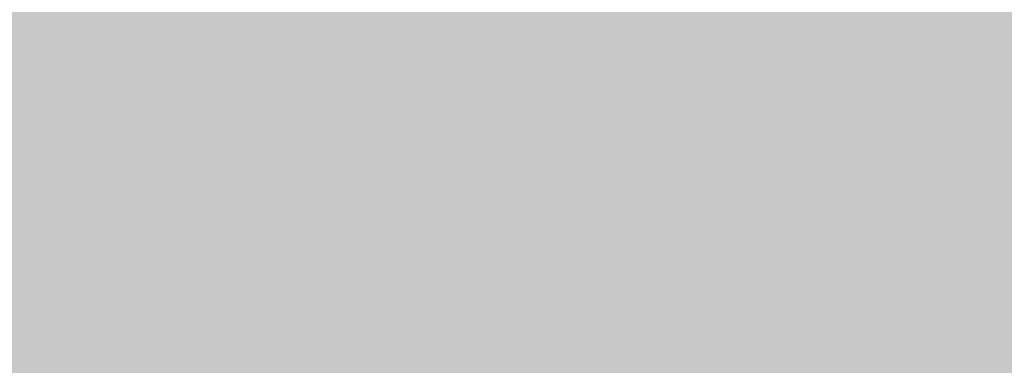
# Model space of a CAD drawing. Units: inches. Extents: x 2091 to 2899, y 967 to 2217.
# Tile 219 of 256: x 2203.2571 to 2203.4104, y 1152.3009 to 1152.3547. Entities that reach past the tile are written whole.
import ezdxf

# ---------------------------------------------------------------- set-up
doc = ezdxf.new("R2010")
doc.units = ezdxf.units.IN
doc.layers.add('A-WALL-PATT', color=141, linetype='Continuous', lineweight=13, true_color=0xadddf7)

msp = doc.modelspace()

# ---------------------------------------------------------------- hatches: boundary and pattern name
at = {"layer": 'A-WALL-PATT'}
h = msp.add_hatch(color=256, dxfattribs=at)
h.dxf.hatch_style = 1
h.paths.add_polyline_path([(2803.1436, 2050.91906), (2203.1436, 2050.91906), (2203.1436, 1090.91906), (2803.1436, 1090.91906)])
h.paths.add_polyline_path([(2635.79885, 1147.54046), (2674.52405, 1147.54046, 0.376086), (2678.52967, 1152.8802), (2678.52967, 1159.55647, 0.333335), (2674.52432, 1163.56185), (2674.52432, 1163.56185), (2674.52432, 1192.93439), (2635.80597, 1192.93439), (2597.08762, 1192.93439), (2597.08762, 1163.56185, 0.333335), (2593.08228, 1159.55647), (2593.08228, 1152.8802, 0.376086), (2597.08789, 1147.54046)], flags=0)
h.paths.add_polyline_path([(2436.01043, 1278.24078, 0.000483), (2435.95264, 1278.21503, -0.001328), (2435.93563, 1278.11169, -0.001711), (2436.11644, 1278.04076, 0.002185)], flags=0)
h.paths.add_polyline_path([(2794.1436, 1143.41906), (2794.1436, 1347.41906), (2543.37017, 1347.41906), (2543.37017, 1351.91906), (2794.1436, 1351.91906), (2794.1436, 1392.71355), (2793.9474, 1392.71355), (2793.9474, 1473.5369), (2794.1436, 1473.5369), (2794.1436, 1531.91906), (2650.1436, 1531.91906), (2650.1436, 1536.41906), (2794.1436, 1536.41906), (2794.1436, 1692.41906), (2609.37561, 1692.41906), (2609.37561, 1644.41906), (2604.87561, 1644.41906), (2604.87561, 1744.91906), (2609.37561, 1744.91906), (2609.37561, 1696.91906), (2794.1436, 1696.91906), (2794.1436, 1780.91906), (2609.6436, 1780.91906), (2493.87561, 1780.91906), (2493.87561, 1785.41906), (2609.6436, 1785.41906), (2794.1436, 1785.41906), (2794.1436, 1847.93882), (2793.95122, 1847.93882), (2793.95122, 1928.76217), (2794.1436, 1928.76217), (2794.1436, 1941.41906), (2614.1436, 1941.41906), (2614.1436, 1821.41906), (2609.6436, 1821.41906), (2609.6436, 1941.41906), (2392.1436, 1941.41906), (2392.1436, 1819.91906), (2387.6436, 1819.91906), (2387.6436, 1941.41906), (2212.1436, 1941.41906), (2212.1436, 1783.91906), (2392.1436, 1783.91906), (2392.1436, 1780.91906), (2212.1436, 1780.91906), (2212.1436, 1629.41906), (2387.6436, 1629.41906), (2387.6436, 1744.91906), (2392.1436, 1744.91906), (2392.1436, 1627.91906), (2317.1436, 1627.91906), (2317.1436, 1551.41906), (2317.1436, 1536.41906), (2459.38359, 1536.41906), (2459.38359, 1602.39648), (2463.88359, 1602.39648), (2463.88359, 1531.91906), (2456.6436, 1531.91906), (2456.6436, 1529.91906), (2452.1436, 1529.91906), (2452.1436, 1531.91906), (2312.6436, 1531.91906), (2312.6436, 1551.41906), (2306.1436, 1551.41906), (2306.1436, 1555.91906), (2308.1436, 1555.91906), (2308.1436, 1551.41906), (2312.6436, 1551.41906), (2312.6436, 1627.91906), (2212.1436, 1627.91906), (2212.1436, 1555.91906), (2270.1436, 1555.91906), (2270.1436, 1551.41906), (2212.1436, 1551.41906), (2212.1436, 1351.91906), (2272.1436, 1351.91906), (2272.1436, 1347.41906), (2212.1436, 1347.41906), (2212.1436, 1275.41906), (2308.1436, 1275.41906), (2308.1436, 1351.91906), (2452.1436, 1351.91906), (2452.1436, 1493.91906), (2456.6436, 1493.91906), (2456.6436, 1347.41906), (2312.6436, 1347.41906), (2312.6436, 1270.91906), (2212.1436, 1270.91906), (2212.1436, 1099.91906), (2281.23752, 1099.91906), (2282.87104, 1110.9138), (2282.00834, 1116.9966), (2278.55774, 1121.4204), (2268.20564, 1128.0562), (2272.08764, 1128.0562), (2273.81294, 1131.927), (2279.42034, 1134.6919), (2285.02784, 1135.2449), (2287.61584, 1137.4568), (2288.04714, 1138.0098), (2289.34114, 1140.7747), (2291.06654, 1139.6687), (2292.36054, 1135.2449), (2295.37984, 1136.9038), (2296.24254, 1135.7979), (2297.10524, 1133.033), (2300.12464, 1138.0098), (2303.14394, 1138.0098), (2304.43794, 1135.7979), (2303.14394, 1133.586), (2306.59464, 1134.6919), (2307.88874, 1133.033), (2310.90804, 1135.2449), (2313.92744, 1134.1389), (2315.62686, 1132.4271), (2308.32004, 1117.5496), (2290.20384, 1109.8079), (2288.90984, 1103.1721), (2289.27231, 1099.91906), (2434.91823, 1099.91906), (2431.59323, 1124.78806), (2429.93023, 1169.55306), (2430.92718, 1240.51969), (2435.65893, 1238.18613), (2437.13523, 1196.55406), (2438.79823, 1143.97306), (2442.67823, 1111.99806), (2446.55823, 1099.91906), (2794.1436, 1099.91906), (2794.1436, 1138.91906), (2548.03245, 1138.91906), (2548.03245, 1143.41906), (2548.03245, 1148.81906), (2546.66846, 1148.03156), (2528.68569, 1179.17862, 0.256256), (2512.03245, 1148.81906), (2512.03245, 1143.41906), (2512.03245, 1138.91906), (2507.53245, 1138.91906), (2507.53245, 1143.41906), (2507.53245, 1148.81906, 0.256256), (2490.8792, 1179.17862), (2472.89644, 1148.03156), (2471.53245, 1148.81906), (2471.53245, 1143.41906), (2467.03245, 1143.41906), (2467.03245, 1269.94579, 0.039061), (2460.90999, 1273.58006), (2467.03245, 1273.58006), (2467.03245, 1286.32536, 0.014511), (2465.21619, 1286.76191), (2467.03245, 1287.05258), (2467.03245, 1323.41906), (2471.53245, 1323.41906), (2471.53245, 1148.81906), (2489.53245, 1179.99597), (2490.89644, 1179.20847), (2490.8792, 1179.17862, -0.256256), (2507.53245, 1148.81906), (2507.53245, 1143.41906), (2512.03245, 1143.41906), (2512.03245, 1148.81906, -0.256256), (2528.68569, 1179.17862), (2528.66846, 1179.20847), (2530.03245, 1179.99597), (2548.03245, 1148.81906), (2548.03245, 1143.41906)], flags=16)
h.paths.add_polyline_path([(2607.76855, 1200.94508), (2607.76855, 1265.03063), (2597.08762, 1281.05201), (2619.78459, 1281.05201), (2627.79528, 1337.12686), (2635.79885, 1337.12686), (2643.81666, 1337.12686), (2651.82736, 1281.05201), (2674.52432, 1281.05201), (2663.8434, 1265.03063), (2663.8434, 1200.94508), (2635.80597, 1200.94508)], flags=0)
edge = h.paths.add_edge_path(flags=0)
edge.add_ellipse((13303.89622, 1272.99872), major_axis=(-10595.31304, 0), ratio=0.84230387009, start_angle=0.628237219, end_angle=0.6465541, ccw=False)
edge.add_ellipse((2711.70045, 1156.85268), major_axis=(2.21977, 0), ratio=0.8423039, start_angle=111.53524, end_angle=180.62824, ccw=False)
edge.add_ellipse((13303.15629, 1272.99872), major_axis=(-10593.02631, 0), ratio=0.84230386954, start_angle=0.528271472, end_angle=0.646554097, ccw=False)
edge.add_line((2710.7646, 1175.3333), (2710.12999, 1175.3333))
edge.add_ellipse((2710.12999, 1176.57978), major_axis=(1.47985, 0), ratio=0.8423039, start_angle=180, end_angle=270, ccw=False)
edge.add_line((2708.65014, 1176.57978), (2708.65014, 1200.78291))
edge.add_ellipse((2710.12999, 1200.78291), major_axis=(1.47985, 0), ratio=0.8423039, start_angle=90, end_angle=180, ccw=False)
edge.add_line((2710.12999, 1202.02939), (2710.46508, 1202.02939))
edge.add_ellipse((13303.15629, 1272.99872), major_axis=(-10593.02631, 0), ratio=0.84230386954, start_angle=-0.090229089, end_angle=0.383866779, ccw=False)
edge.add_ellipse((2710.12999, 1290.92703), major_axis=(-1.47985, 0), ratio=0.8423039, start_angle=0, end_angle=90, ccw=False)
edge.add_line((2708.65014, 1290.92703), (2708.65014, 1315.13017))
edge.add_ellipse((2710.12999, 1315.13017), major_axis=(-1.47985, 0), ratio=0.8423039, start_angle=-90, end_angle=0, ccw=False)
edge.add_line((2710.12999, 1316.37665), (2710.70631, 1316.37665))
edge.add_ellipse((3238.40172, 1296.28957), major_axis=(528.234, 0), ratio=0.84230387, start_angle=176.3495724, end_angle=177.8200497, ccw=False)
edge.add_ellipse((2775.06304, 1071.4507), major_axis=(313.30776, 0), ratio=0.84230387, start_angle=102.1259656, end_angle=103.780529, ccw=False)
edge.add_ellipse((2775.06304, 1078.3057), major_axis=(-305.30289, 0), ratio=0.84230387, start_angle=-79.790461, end_angle=-77.5553727, ccw=False)
edge.add_ellipse((2695.14177, 1541.97538), major_axis=(-250.96022, 0), ratio=0.84230387, start_angle=99.256566, end_angle=102.5549326)
edge.add_line((2741.41033, 1334.21426), (2747.13255, 1337.37848))
edge.add_ellipse((2747.53862, 1336.85748), major_axis=(-0.73992, 0), ratio=0.842304, start_angle=270, end_angle=307.93313, ccw=False)
edge.add_ellipse((2747.53862, 1336.85748), major_axis=(-0.73992, 0), ratio=0.842304, start_angle=232.06687, end_angle=270, ccw=False)
edge.add_line((2747.94469, 1337.37848), (2753.66691, 1334.21426))
edge.add_ellipse((2799.93547, 1541.97538), major_axis=(250.96022, 0), ratio=0.84230387, start_angle=257.4450674, end_angle=260.743434)
edge.add_ellipse((2720.01419, 1078.3057), major_axis=(305.30289, 0), ratio=0.84230387, start_angle=77.5553727, end_angle=79.790461, ccw=False)
edge.add_ellipse((2720.01419, 1071.4507), major_axis=(-313.30776, 0), ratio=0.84230387, start_angle=256.219471, end_angle=257.8740344, ccw=False)
edge.add_ellipse((2256.67551, 1296.28957), major_axis=(-528.234, 0), ratio=0.84230387, start_angle=182.1799503, end_angle=183.6504276, ccw=False)
edge.add_line((2784.37092, 1316.37665), (2784.94725, 1316.37665))
edge.add_ellipse((2784.94725, 1315.13017), major_axis=(1.47985, 0), ratio=0.8423039, start_angle=0, end_angle=90, ccw=False)
edge.add_line((2786.42709, 1315.13017), (2786.42709, 1290.92703))
edge.add_ellipse((2784.94725, 1290.92703), major_axis=(1.47985, 0), ratio=0.8423039, start_angle=270, end_angle=360, ccw=False)
edge.add_ellipse((-7808.07906, 1272.99872), major_axis=(10593.02631, 0), ratio=0.84230386954, start_angle=-0.383866779, end_angle=0.090229089, ccw=False)
edge.add_line((2784.61216, 1202.02939), (2784.94725, 1202.02939))
edge.add_ellipse((2784.94725, 1200.78291), major_axis=(1.47985, 0), ratio=0.8423039, start_angle=0, end_angle=90, ccw=False)
edge.add_line((2786.42709, 1200.78291), (2786.42709, 1176.57978))
edge.add_ellipse((2784.94725, 1176.57978), major_axis=(-1.47985, 0), ratio=0.8423039, start_angle=90, end_angle=180, ccw=False)
edge.add_line((2784.94725, 1175.3333), (2784.31264, 1175.3333))
edge.add_ellipse((-7808.07906, 1272.99872), major_axis=(10593.02631, 0), ratio=0.84230386954, start_angle=-0.618643196, end_angle=-0.528271472, ccw=False)
edge.add_ellipse((2783.37678, 1156.85268), major_axis=(-2.21977, 0), ratio=0.8423039, start_angle=179.37176, end_angle=248.46476, ccw=False)
edge.add_ellipse((-7808.81898, 1272.99872), major_axis=(-10595.31304, 0), ratio=0.84230386576, start_angle=179.353445923, end_angle=179.371762803, ccw=False)
edge.add_ellipse((2780.2973, 1153.50079), major_axis=(-5.24643, 0), ratio=0.8423039, start_angle=90, end_angle=179.35345, ccw=False)
edge.add_line((2780.2973, 1149.08171), (2714.77993, 1149.08171))
edge.add_ellipse((2714.77993, 1153.50079), major_axis=(5.24643, 0), ratio=0.8423039, start_angle=180.64655, end_angle=270, ccw=False)
edge = h.paths.add_edge_path(flags=0)
edge.add_line((2718.18737, 1151.00783), (2718.18737, 1170.47236))
edge.add_ellipse((2721.14706, 1170.47236), major_axis=(-2.95969, 0), ratio=0.8423039, start_angle=-90, end_angle=0, ccw=False)
edge.add_line((2721.14706, 1172.96532), (2773.93017, 1172.96532))
edge.add_ellipse((2773.93017, 1170.47236), major_axis=(-2.95969, 0), ratio=0.8423039, start_angle=180, end_angle=270, ccw=False)
edge.add_line((2776.88987, 1170.47236), (2776.88987, 1151.00783))
edge.add_line((2776.88987, 1151.00783), (2718.18737, 1151.00783))
edge = h.paths.add_edge_path(flags=0)
edge.add_line((2718.18737, 1180.23415), (2718.18737, 1199.05783))
edge.add_ellipse((2747.53862, 1320.39864), major_axis=(147.01792, 0), ratio=0.84230387, start_angle=256.4018653, end_angle=283.5981347)
edge.add_line((2776.88987, 1199.05783), (2776.88987, 1180.23415))
edge.add_ellipse((2747.53862, 1301.57496), major_axis=(147.01792, 0), ratio=0.84230387, start_angle=256.4018653, end_angle=283.5981347, ccw=False)
edge = h.paths.add_edge_path(flags=0)
edge.add_ellipse((13303.15629, 1272.99872), major_axis=(-10591.54646, 0), ratio=0.84230386955, start_angle=0.055594314, end_angle=0.377764194, ccw=False)
edge.add_line((2711.61686, 1262.72171), (2715.66741, 1249.4954))
edge.add_ellipse((6413.89196, 1241.69192), major_axis=(-3698.23616, 0), ratio=0.8423038695, start_angle=-0.12089737, end_angle=0.36407635)
edge.add_line((2715.76104, 1218.19245), (2711.93431, 1203.16736))
edge = h.paths.add_edge_path(flags=0)
edge.add_line((2718.18737, 1251.07457), (2716.00249, 1267.45044))
edge.add_ellipse((2742.15117, 1202.18954), major_axis=(81.77258, 0), ratio=0.84230387, start_angle=94.277421, end_angle=111.8349538, ccw=False)
edge.add_line((2737.00975, 1270.93063), (2758.06748, 1270.93063))
edge.add_ellipse((2752.92606, 1202.18954), major_axis=(81.77258, 0), ratio=0.84230387, start_angle=68.1650462, end_angle=85.722579, ccw=False)
edge.add_line((2779.07475, 1267.45044), (2776.88987, 1251.07457))
edge.add_ellipse((2750.33806, 1187.88536), major_axis=(79.57966, 0), ratio=0.84230387, start_angle=67.2080851, end_angle=85.1299304)
edge.add_line((2756.03466, 1254.74366), (2739.04258, 1254.74366))
edge.add_ellipse((2744.73917, 1187.88536), major_axis=(79.57966, 0), ratio=0.84230387, start_angle=94.8700696, end_angle=112.7919149)
edge = h.paths.add_edge_path(flags=0)
edge.add_line((2783.14293, 1203.16736), (2779.31619, 1218.19245))
edge.add_ellipse((-918.81473, 1241.69192), major_axis=(3698.23616, 0), ratio=0.8423038695, start_angle=-0.36407635, end_angle=0.12089737)
edge.add_line((2779.40983, 1249.4954), (2783.46037, 1262.72171))
edge.add_ellipse((-7808.07906, 1272.99872), major_axis=(-10591.54646, 0), ratio=0.84230386954, start_angle=179.622235806, end_angle=179.944405687, ccw=False)
edge = h.paths.add_edge_path(flags=0)
edge.add_ellipse((2734.20089, 1286.69044), major_axis=(-0.35661, 6.34008), ratio=0.6038336, start_angle=89.002014, end_angle=253.657408, ccw=False)
edge.add_line((2730.369, 1286.54181), (2730.369, 1301.35198))
edge.add_line((2730.369, 1301.35198), (2735.91331, 1305.2148))
edge.add_ellipse((2736.38492, 1304.73456), major_axis=(0.73992, 0), ratio=0.842304, start_angle=90, end_angle=134.48021, ccw=False)
edge.add_line((2736.38492, 1305.3578), (2738.03278, 1305.3578))
edge.add_line((2738.03278, 1305.3578), (2738.03278, 1307.70793))
edge.add_ellipse((2794.20164, 1307.70793), major_axis=(56.16886, 0), ratio=0.84230387, start_angle=150.56143, end_angle=180, ccw=False)
edge.add_ellipse((2700.87559, 1307.70793), major_axis=(-56.16886, 0), ratio=0.84230387, start_angle=180, end_angle=209.43857, ccw=False)
edge.add_line((2757.04445, 1307.70793), (2757.04445, 1305.3578))
edge.add_line((2757.04445, 1305.3578), (2758.69232, 1305.3578))
edge.add_ellipse((2758.69232, 1304.73456), major_axis=(-0.73992, 0), ratio=0.842304, start_angle=225.51979, end_angle=270, ccw=False)
edge.add_line((2759.16392, 1305.2148), (2764.70823, 1301.35198))
edge.add_line((2764.70823, 1301.35198), (2764.70823, 1286.54181))
edge.add_ellipse((2760.87634, 1286.69044), major_axis=(0.35661, 6.34008), ratio=0.6038336, start_angle=106.342592, end_angle=270.997986, ccw=False)
edge.add_line((2757.04445, 1285.79709), (2757.04445, 1307.70793))
edge.add_ellipse((2700.87559, 1307.70793), major_axis=(-56.16886, 0), ratio=0.84230387, start_angle=180, end_angle=209.43857)
edge.add_ellipse((2794.20164, 1307.70793), major_axis=(56.16886, 0), ratio=0.84230387, start_angle=150.56143, end_angle=180)
edge.add_line((2738.03278, 1307.70793), (2738.03278, 1285.79709))
h.paths.add_polyline_path([(2417.81227, 1104.4497), (2413.49227, 1102.5297), (2410.61227, 1103.9697), (2409.17227, 1106.3697), (2407.25227, 1107.3297), (2406.29227, 1109.7297), (2405.33227, 1114.0497), (2405.33227, 1117.8897), (2406.29227, 1120.1297), (2407.25227, 1119.8097), (2408.84832, 1118.32766), (2410.17395, 1119.42417), (2410.21127, 1120.4057), (2411.04073, 1121.41905), (2410.69927, 1119.8587), (2410.17395, 1119.42417), (2410.08845, 1117.17611), (2411.13284, 1116.20632), (2413.97227, 1119.3297), (2416.85227, 1120.7697), (2416.86972, 1120.79878), (2417.03507, 1119.40512), (2417.89621, 1118.14338), (2418.29227, 1118.3697), (2419.54445, 1120.03927), (2419.36092, 1118.38749), (2419.03211, 1119.35615), (2418.39894, 1118.51193), (2419.25227, 1114.5297), (2418.79409, 1107.19879)], flags=0)
h.paths.add_polyline_path([(2508.87017, 1347.41906), (2508.37017, 1347.41906), (2508.37017, 1351.91906), (2508.87017, 1351.91906)], flags=0)
h.paths.add_polyline_path([(2473.37017, 1347.41906), (2472.37017, 1347.41906), (2467.87017, 1347.41906), (2467.87017, 1455.41906), (2472.37017, 1455.41906), (2472.37017, 1352.41906), (2473.37017, 1352.41906)], flags=0)
h.paths.add_polyline_path([(2352.10624, 1217.4462), (2349.22624, 1218.8862), (2347.78624, 1221.2862), (2345.86624, 1222.2462), (2344.90624, 1224.6462), (2343.94624, 1228.9662), (2343.94624, 1232.8062), (2344.90624, 1235.0462), (2345.86624, 1234.7262), (2347.46229, 1233.24415), (2348.78792, 1234.34066), (2348.82524, 1235.3222), (2349.6547, 1236.33555), (2349.31324, 1234.7752), (2348.78792, 1234.34066), (2348.70242, 1232.0926), (2349.74681, 1231.12282), (2352.58624, 1234.2462), (2355.46624, 1235.6862), (2355.48369, 1235.71528), (2355.64904, 1234.32161), (2356.51018, 1233.05988), (2356.90624, 1233.2862), (2358.15842, 1234.95576), (2357.97489, 1233.30398), (2357.64608, 1234.27264), (2357.01291, 1233.42842), (2357.86624, 1229.4462), (2357.40806, 1222.11529), (2356.42624, 1219.3662)], flags=0)
h.paths.add_polyline_path([(2348.2968, 1112.22442), (2347.0138, 1112.31042), (2345.5298, 1114.12742), (2345.7318, 1115.85842), (2346.8118, 1116.98242), (2346.8118, 1114.64642), (2345.8668, 1114.21442), (2346.8798, 1114.30042)], flags=0)
h.paths.add_polyline_path([(2347.0138, 1110.92642), (2346.2718, 1110.49342), (2346.6098, 1111.18642)], flags=0)
h.paths.add_polyline_path([(2345.8668, 1118.19442), (2345.5298, 1117.32942), (2343.7078, 1118.02142), (2344.3828, 1118.62642)], flags=0)
h.paths.add_polyline_path([(2346.6768, 1109.28242), (2346.0698, 1108.07142), (2345.8668, 1110.06142)], flags=0)
h.paths.add_polyline_path([(2345.0568, 1119.75142), (2343.6398, 1119.75142), (2343.9778, 1121.13542)], flags=0)
h.paths.add_polyline_path([(2345.2598, 1116.55042), (2345.1248, 1115.85842), (2344.9218, 1115.68542), (2344.7198, 1116.37742)], flags=0)
h.paths.add_polyline_path([(2345.6648, 1112.31042), (2345.4618, 1111.53242), (2344.0448, 1111.96442), (2344.6518, 1112.57042)], flags=0)
h.paths.add_polyline_path([(2345.1918, 1113.34942), (2344.4498, 1113.86842), (2344.7198, 1114.38742)], flags=0)
h.paths.add_polyline_path([(2344.6518, 1116.80942), (2344.1798, 1115.68542), (2344.6518, 1115.33942), (2343.9098, 1114.90642), (2343.0328, 1115.94442), (2343.6398, 1116.46342)], flags=0)
h.paths.add_polyline_path([(2345.8668, 1106.68642), (2344.9898, 1105.56242), (2344.5168, 1106.60042)], flags=0)
h.paths.add_polyline_path([(2344.8548, 1110.06142), (2344.5168, 1109.28242), (2344.1128, 1109.71542)], flags=0)
h.paths.add_polyline_path([(2344.0448, 1113.52242), (2343.4378, 1113.08942), (2342.7628, 1113.95442)], flags=0)
h.paths.add_polyline_path([(2344.3148, 1111.01242), (2342.9648, 1110.32042), (2342.9648, 1111.09942)], flags=0)
h.paths.add_polyline_path([(2345.1248, 1104.69742), (2344.5848, 1103.74542), (2344.4498, 1104.26442)], flags=0)
h.paths.add_polyline_path([(2342.8298, 1121.22242), (2341.7498, 1120.53042), (2340.5358, 1121.04942), (2340.1308, 1121.82842), (2340.6708, 1122.95242), (2341.1428, 1121.82842), (2341.6148, 1122.00142)], flags=0)
h.paths.add_polyline_path([(2342.9648, 1119.75142), (2343.0328, 1118.45342), (2342.0878, 1118.02142), (2342.0198, 1119.49142)], flags=0)
h.paths.add_polyline_path([(2342.6948, 1116.89642), (2341.9528, 1116.63642), (2342.0198, 1117.32942)], flags=0)
h.paths.add_polyline_path([(2343.0328, 1112.22442), (2342.0198, 1111.79142), (2341.5478, 1112.22442), (2342.3578, 1113.34942)], flags=0)
h.paths.add_polyline_path([(2343.7748, 1104.43742), (2342.6278, 1102.88042), (2342.6948, 1104.61042), (2343.4378, 1105.12942)], flags=0)
h.paths.add_polyline_path([(2342.0198, 1115.07942), (2340.8058, 1115.51242), (2340.9408, 1116.37742)], flags=0)
h.paths.add_polyline_path([(2341.4808, 1120.09742), (2341.4808, 1119.40542), (2341.0758, 1119.57842), (2341.1428, 1120.09742)], flags=0)
h.paths.add_polyline_path([(2341.8178, 1114.47342), (2340.9408, 1113.08942), (2340.8058, 1114.56042)], flags=0)
h.paths.add_polyline_path([(2341.1428, 1118.54042), (2340.9408, 1116.98242), (2339.0508, 1117.67542), (2339.0508, 1118.62642)], flags=0)
h.paths.add_polyline_path([(2342.6948, 1101.66842), (2341.9528, 1101.84142), (2342.5598, 1102.36142)], flags=0)
h.paths.add_polyline_path([(2340.3328, 1119.66542), (2338.4438, 1119.57842), (2337.9038, 1120.35742), (2339.6578, 1120.61642)], flags=0)
h.paths.add_polyline_path([(2340.3328, 1115.33942), (2340.0628, 1113.69542), (2339.3878, 1115.33942)], flags=0)
h.paths.add_polyline_path([(2341.8178, 1103.83142), (2341.5478, 1102.88042), (2341.1428, 1103.65842)], flags=0)
h.paths.add_polyline_path([(2339.0508, 1122.86642), (2337.2958, 1121.82842), (2337.0938, 1123.12542), (2337.7688, 1123.81842)], flags=0)
h.paths.add_polyline_path([(2339.1178, 1121.74142), (2338.8478, 1121.22242), (2338.1738, 1121.04942), (2338.3758, 1121.56842)], flags=0)
h.paths.add_polyline_path([(2339.1858, 1119.31942), (2338.6458, 1118.71342), (2338.2408, 1118.10742), (2338.2408, 1118.88642)], flags=0)
h.paths.add_polyline_path([(2341.1428, 1101.92842), (2340.6028, 1101.23642), (2340.0628, 1101.84142), (2340.6028, 1102.36142)], flags=0)
h.paths.add_polyline_path([(2337.6338, 1117.76142), (2336.6208, 1118.28042), (2337.2958, 1118.97242)], flags=0)
h.paths.add_polyline_path([(2336.8238, 1119.57842), (2334.7988, 1118.97242), (2335.2038, 1120.35742), (2336.5538, 1120.87642)], flags=0)
h.paths.add_polyline_path([(2339.1178, 1100.45742), (2337.3638, 1100.54342), (2336.7558, 1101.23642)], flags=0)
h.paths.add_polyline_path([(2336.3508, 1122.43342), (2336.0138, 1121.91442), (2334.9338, 1122.43342), (2334.5288, 1123.47142), (2335.7438, 1122.77942)], flags=0)
h.paths.add_polyline_path([(2334.7318, 1120.87642), (2334.2588, 1120.35742), (2334.0568, 1120.78942), (2334.5968, 1121.30842)], flags=0)
h.paths.add_polyline_path([(2334.4618, 1122.17442), (2332.5718, 1121.30842), (2331.3568, 1122.17442), (2332.0998, 1122.86642)], flags=0)
h.paths.add_polyline_path([(2334.2588, 1118.54042), (2333.3818, 1118.45342), (2333.6518, 1119.31942)], flags=0)
h.paths.add_polyline_path([(2335.5418, 1102.27442), (2334.1918, 1102.62042), (2335.2718, 1103.31242)], flags=0)
h.paths.add_polyline_path([(2332.7068, 1119.66542), (2331.6948, 1120.44342), (2332.5048, 1120.78942)], flags=0)
h.paths.add_polyline_path([(2334.7318, 1101.14942), (2333.5168, 1101.58242), (2333.9888, 1101.75542)], flags=0)
h.paths.add_polyline_path([(2332.6398, 1116.63642), (2331.0868, 1116.29042), (2331.9648, 1118.19442)], flags=0)
h.paths.add_polyline_path([(2330.7498, 1121.56842), (2330.2768, 1120.27042), (2328.5228, 1119.31942), (2328.9948, 1121.04942)], flags=0)
h.paths.add_polyline_path([(2330.7498, 1118.62642), (2330.0078, 1117.50242), (2329.8728, 1118.02142)], flags=0)
h.paths.add_polyline_path([(2332.0998, 1102.36142), (2330.5468, 1102.01442), (2331.6948, 1102.96642)], flags=0)
h.paths.add_polyline_path([(2329.5348, 1113.60842), (2329.0628, 1112.31042), (2328.5898, 1113.34942)], flags=0)
h.paths.add_polyline_path([(2328.3878, 1117.84842), (2327.5098, 1116.55042), (2327.1728, 1117.76142)], flags=0)
h.paths.add_polyline_path([(2329.7378, 1106.51342), (2329.5348, 1105.30242), (2328.2528, 1106.08142)], flags=0)
h.paths.add_polyline_path([(2328.6578, 1114.38742), (2328.0498, 1114.12742), (2328.3198, 1114.90642)], flags=0)
h.paths.add_polyline_path([(2328.3198, 1112.22442), (2327.1058, 1112.13742), (2326.7008, 1112.65642)], flags=0)
h.paths.add_polyline_path([(2326.9028, 1115.25242), (2326.7008, 1114.12742), (2325.2158, 1113.60842), (2326.0928, 1115.33942)], flags=0)
h.paths.add_polyline_path([(2326.6328, 1108.33042), (2326.0928, 1107.37942), (2325.8908, 1108.50342), (2326.4978, 1109.10942)], flags=0)
h.paths.add_polyline_path([(2615.1436, 1531.91906), (2609.6436, 1531.91906), (2609.6436, 1620.41906), (2614.1436, 1620.41906), (2614.1436, 1536.41906), (2615.1436, 1536.41906)], flags=0)
h.paths.add_polyline_path([(2545.1436, 1563.41906), (2464.1436, 1563.41906), (2464.1436, 1632.41906), (2509.1436, 1632.41906), (2509.1436, 1627.91906), (2509.1436, 1603.91906), (2468.6436, 1603.91906), (2468.6436, 1567.91906), (2540.6436, 1567.91906), (2540.6436, 1591.91906), (2545.1436, 1591.91906)], flags=0)
h.paths.add_polyline_path([(2388.96905, 1549.98573), (2357.43418, 1549.98573), (2357.43418, 1623.36078), (2399.36278, 1623.36078), (2435.68947, 1623.36078), (2435.59255, 1602.55927), (2435.59255, 1602.39648), (2388.96905, 1602.39648)], flags=0)
h.paths.add_polyline_path([(2388.88063, 1555.80915), (2374.90443, 1555.80915), (2374.90443, 1600.57156), (2374.90443, 1615.45765), (2406.35088, 1615.45765), (2406.35088, 1618.93943), (2412.17429, 1615.45765), (2406.35088, 1611.97586), (2406.35088, 1615.45765), (2388.88063, 1615.45765)], flags=0)
h.paths.add_polyline_path([(2568.87561, 1644.41906), (2453.37561, 1644.41906), (2453.37561, 1785.41906), (2457.87561, 1785.41906), (2457.87561, 1648.91906), (2568.87561, 1648.91906)], flags=0)
h.paths.add_polyline_path([(2212.1436, 1945.91906), (2212.1436, 2041.91906), (2794.1436, 2041.91906), (2794.1436, 1945.91906)], flags=16)
h.paths.add_polyline_path([(2271.08273, 1964.31724), (2776.85297, 1964.31724), (2776.85297, 2037.16962), (2271.08273, 2037.16962)], flags=8)
h.paths.add_polyline_path([(2380.64929, 1536.82414), (2461.04081, 1536.82414), (2461.04081, 1554.65259), (2380.64929, 1554.65259)], flags=8)
h.paths.add_polyline_path([(2240.75571, 1609.72545), (2309.18583, 1609.72545), (2309.18583, 1617.6982), (2240.75571, 1617.6982)], flags=8)
h.paths.add_polyline_path([(2212.67726, 1313.5041), (2282.59152, 1313.5041), (2282.59152, 1322.74524), (2212.67726, 1322.74524)], flags=8)
h.paths.add_polyline_path([(2457.11198, 1114.77857), (2558.48158, 1114.77857), (2558.48158, 1142.21968), (2457.11198, 1142.21968)], flags=8)
h.paths.add_polyline_path([(2473.44234, 1273.01007), (2604.64123, 1273.01007), (2604.64123, 1318.34693), (2473.44234, 1318.34693)], flags=8)
h.paths.add_polyline_path([(2638.8763, 1626.97743), (2684.25037, 1627.97674), (2684.03848, 1637.59749), (2638.66442, 1636.59819)], flags=8)
h.paths.add_polyline_path([(2537.59055, 1453.79345), (2628.38955, 1453.79345), (2628.38955, 1475.34481), (2537.59055, 1475.34481)], flags=8)
h.paths.add_polyline_path([(2504.13764, 1714.6324), (2554.64719, 1714.6324), (2554.64719, 1730.23771), (2504.13764, 1730.23771)], flags=8)
h.paths.add_polyline_path([(2487.50118, 1575.65187), (2535.09712, 1575.65187), (2535.09712, 1598.37765), (2487.50118, 1598.37765)], flags=8)
h.paths.add_polyline_path([(2709.0994, 1735.71028), (2740.0166, 1735.71028), (2740.0166, 1749.93764), (2709.0994, 1749.93764)], flags=8)
h.paths.add_polyline_path([(2442.43842, 1792.17166), (2564.72884, 1792.17166), (2564.72884, 1842.00016), (2442.43842, 1842.00016)], flags=8)
h.paths.add_polyline_path([(2655.8158, 1809.64408), (2789.52014, 1806.6938), (2790.08498, 1832.29164), (2656.38064, 1835.24192)], flags=8)
h.paths.add_polyline_path([(2234.8427, 1797.72014), (2368.59285, 1794.76885), (2369.16072, 1820.50413), (2235.41056, 1823.45542)], flags=8)
h.paths.add_polyline_path([(2245.13847, 1644.00633), (2398.42773, 1640.6239), (2398.99484, 1666.32482), (2245.70557, 1669.70725)], flags=8)
h.paths.add_polyline_path([(2306.14285, 1431.16852), (2413.76831, 1428.79369), (2414.33315, 1454.39153), (2306.70768, 1456.76636)], flags=8)
h.paths.add_polyline_path([(2306.83458, 1458.23314), (2393.38048, 1456.32345), (2393.93281, 1481.35436), (2307.38691, 1483.26405)], flags=8)

doc.saveas('drawing.dxf')
